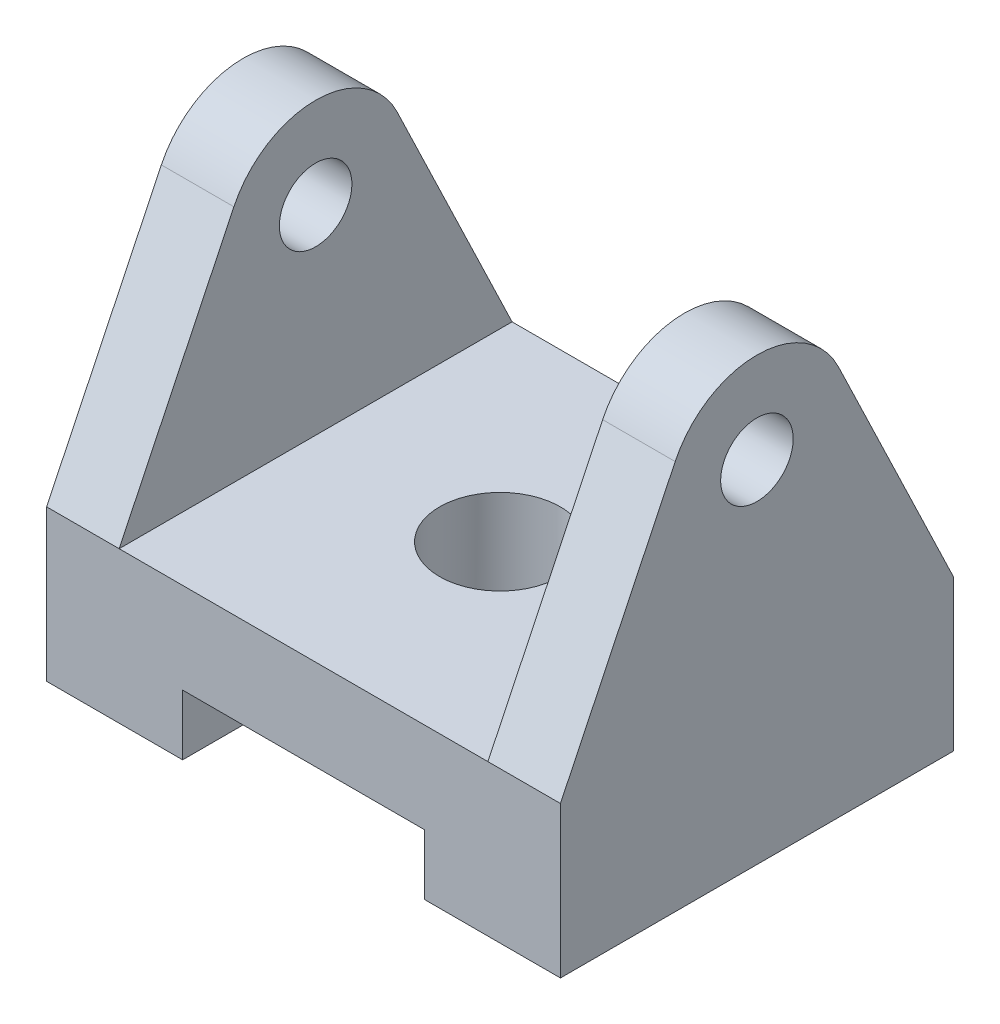
ISO-10303-21;
HEADER;
FILE_DESCRIPTION(('STEP AP214'),'2;1');
FILE_NAME('part.step','',(''),(''),'','','');
FILE_SCHEMA(('AUTOMOTIVE_DESIGN { 1 0 10303 214 1 1 1 1 }'));
ENDSEC;
DATA;
#1=APPLICATION_CONTEXT('core data for automotive mechanical design processes');
#2=APPLICATION_PROTOCOL_DEFINITION('international standard','automotive_design',2000,#1);
#3=PRODUCT_CONTEXT('',#1,'mechanical');
#4=PRODUCT('Part','Part','',(#3));
#5=PRODUCT_RELATED_PRODUCT_CATEGORY('part','',(#4));
#6=PRODUCT_DEFINITION_FORMATION('','',#4);
#7=PRODUCT_DEFINITION_CONTEXT('part definition',#1,'design');
#8=PRODUCT_DEFINITION('design','',#6,#7);
#9=PRODUCT_DEFINITION_SHAPE('','',#8);
#10=(LENGTH_UNIT() NAMED_UNIT(*) SI_UNIT(.MILLI.,.METRE.));
#11=(NAMED_UNIT(*) PLANE_ANGLE_UNIT() SI_UNIT($,.RADIAN.));
#12=(NAMED_UNIT(*) SI_UNIT($,.STERADIAN.) SOLID_ANGLE_UNIT());
#13=UNCERTAINTY_MEASURE_WITH_UNIT(LENGTH_MEASURE(1.E-05),#10,'distance_accuracy_value','');
#14=(GEOMETRIC_REPRESENTATION_CONTEXT(3) GLOBAL_UNCERTAINTY_ASSIGNED_CONTEXT((#13)) GLOBAL_UNIT_ASSIGNED_CONTEXT((#10,
#11,#12)) REPRESENTATION_CONTEXT('',''));
#15=CARTESIAN_POINT('',(0.,0.,0.));
#16=DIRECTION('',(0.,0.,1.));
#17=DIRECTION('',(1.,0.,0.));
#18=AXIS2_PLACEMENT_3D('',#15,#16,#17);
#19=CARTESIAN_POINT('',(30.5,29.,32.5));
#20=DIRECTION('',(1.,0.,0.));
#21=DIRECTION('',(0.,0.,-1.));
#22=AXIS2_PLACEMENT_3D('',#19,#20,#21);
#23=PLANE('',#22);
#24=CARTESIAN_POINT('',(30.5,29.,0.));
#25=DIRECTION('',(1.,0.,0.));
#26=DIRECTION('',(0.,1.,0.));
#27=AXIS2_PLACEMENT_3D('',#24,#25,#26);
#28=CIRCLE('',#27,6.);
#29=CARTESIAN_POINT('',(30.5,35.,0.));
#30=VERTEX_POINT('',#29);
#31=EDGE_CURVE('E193',#30,#30,#28,.T.);
#32=ORIENTED_EDGE('',*,*,#31,.T.);
#33=EDGE_LOOP('',(#32));
#34=FACE_BOUND('',#33,.T.);
#35=DIRECTION('',(0.,0.,-1.));
#36=VECTOR('',#35,1.);
#37=CARTESIAN_POINT('',(30.5,-4.,32.5));
#38=LINE('',#37,#36);
#39=CARTESIAN_POINT('',(30.5,-4.,32.5));
#40=VERTEX_POINT('',#39);
#41=CARTESIAN_POINT('',(30.5,-4.,-32.5));
#42=VERTEX_POINT('',#41);
#43=EDGE_CURVE('E51',#40,#42,#38,.T.);
#44=ORIENTED_EDGE('',*,*,#43,.F.);
#45=DIRECTION('',(0.,0.901331634338171,-0.433129639878502));
#46=VECTOR('',#45,1.);
#47=CARTESIAN_POINT('',(30.5,11.9373818614747,24.8413844546404));
#48=LINE('',#47,#46);
#49=CARTESIAN_POINT('',(30.5,35.4969445981775,13.5199745150726));
#50=VERTEX_POINT('',#49);
#51=EDGE_CURVE('E198',#40,#50,#48,.T.);
#52=ORIENTED_EDGE('',*,*,#51,.T.);
#53=CARTESIAN_POINT('',(30.5,29.,0.));
#54=DIRECTION('',(1.,0.,0.));
#55=DIRECTION('',(0.,1.,0.));
#56=AXIS2_PLACEMENT_3D('',#53,#54,#55);
#57=CIRCLE('',#56,15.);
#58=CARTESIAN_POINT('',(30.5,35.4969445981775,-13.5199745150726));
#59=VERTEX_POINT('',#58);
#60=EDGE_CURVE('E192',#59,#50,#57,.T.);
#61=ORIENTED_EDGE('',*,*,#60,.F.);
#62=DIRECTION('',(0.,0.901331634338171,0.433129639878502));
#63=VECTOR('',#62,1.);
#64=CARTESIAN_POINT('',(30.5,11.9373818614747,-24.8413844546404));
#65=LINE('',#64,#63);
#66=EDGE_CURVE('E186',#42,#59,#65,.T.);
#67=ORIENTED_EDGE('',*,*,#66,.F.);
#68=EDGE_LOOP('',(#44,#52,#61,#67));
#69=FACE_BOUND('',#68,.T.);
#70=ADVANCED_FACE('F41',(#34,#69),#23,.F.);
#71=CARTESIAN_POINT('',(-30.5,29.,32.5));
#72=DIRECTION('',(-1.,0.,0.));
#73=DIRECTION('',(0.,0.,1.));
#74=AXIS2_PLACEMENT_3D('',#71,#72,#73);
#75=PLANE('',#74);
#76=CARTESIAN_POINT('',(-30.5,29.,0.));
#77=DIRECTION('',(-1.,0.,0.));
#78=DIRECTION('',(0.,0.,1.));
#79=AXIS2_PLACEMENT_3D('',#76,#77,#78);
#80=CIRCLE('',#79,6.);
#81=CARTESIAN_POINT('',(-30.5,29.,6.));
#82=VERTEX_POINT('',#81);
#83=EDGE_CURVE('E203',#82,#82,#80,.T.);
#84=ORIENTED_EDGE('',*,*,#83,.T.);
#85=EDGE_LOOP('',(#84));
#86=FACE_BOUND('',#85,.T.);
#87=DIRECTION('',(0.,0.901331634338171,-0.433129639878502));
#88=VECTOR('',#87,1.);
#89=CARTESIAN_POINT('',(-30.5,11.9373818614747,24.8413844546404));
#90=LINE('',#89,#88);
#91=CARTESIAN_POINT('',(-30.5,-4.00000000000002,32.5));
#92=VERTEX_POINT('',#91);
#93=CARTESIAN_POINT('',(-30.5,35.4969445981775,13.5199745150726));
#94=VERTEX_POINT('',#93);
#95=EDGE_CURVE('E577',#92,#94,#90,.T.);
#96=ORIENTED_EDGE('',*,*,#95,.F.);
#97=DIRECTION('',(0.,0.,-1.));
#98=VECTOR('',#97,1.);
#99=CARTESIAN_POINT('',(-30.5,-4.,32.5));
#100=LINE('',#99,#98);
#101=CARTESIAN_POINT('',(-30.5,-4.,-32.5));
#102=VERTEX_POINT('',#101);
#103=EDGE_CURVE('E151',#92,#102,#100,.T.);
#104=ORIENTED_EDGE('',*,*,#103,.T.);
#105=DIRECTION('',(0.,0.901331634338172,0.433129639878502));
#106=VECTOR('',#105,1.);
#107=CARTESIAN_POINT('',(-30.5,11.9373818614747,-24.8413844546404));
#108=LINE('',#107,#106);
#109=CARTESIAN_POINT('',(-30.5,35.4969445981775,-13.5199745150726));
#110=VERTEX_POINT('',#109);
#111=EDGE_CURVE('E602',#102,#110,#108,.T.);
#112=ORIENTED_EDGE('',*,*,#111,.T.);
#113=CARTESIAN_POINT('',(-30.5,29.,0.));
#114=DIRECTION('',(-1.,0.,0.));
#115=DIRECTION('',(0.,-1.,0.));
#116=AXIS2_PLACEMENT_3D('',#113,#114,#115);
#117=CIRCLE('',#116,15.);
#118=EDGE_CURVE('E578',#110,#94,#117,.F.);
#119=ORIENTED_EDGE('',*,*,#118,.T.);
#120=EDGE_LOOP('',(#96,#104,#112,#119));
#121=FACE_BOUND('',#120,.T.);
#122=ADVANCED_FACE('F268',(#86,#121),#75,.F.);
#123=CARTESIAN_POINT('',(20.,-29.,32.5));
#124=DIRECTION('',(0.,1.,0.));
#125=DIRECTION('',(0.,0.,1.));
#126=AXIS2_PLACEMENT_3D('',#123,#124,#125);
#127=PLANE('',#126);
#128=DIRECTION('',(1.,0.,0.));
#129=VECTOR('',#128,1.);
#130=CARTESIAN_POINT('',(20.,-29.,-32.5));
#131=LINE('',#130,#129);
#132=CARTESIAN_POINT('',(20.,-29.,-32.5));
#133=VERTEX_POINT('',#132);
#134=CARTESIAN_POINT('',(42.5,-29.,-32.5));
#135=VERTEX_POINT('',#134);
#136=EDGE_CURVE('E131',#133,#135,#131,.T.);
#137=ORIENTED_EDGE('',*,*,#136,.T.);
#138=DIRECTION('',(0.,0.,-1.));
#139=VECTOR('',#138,1.);
#140=CARTESIAN_POINT('',(42.5,-29.,32.5));
#141=LINE('',#140,#139);
#142=CARTESIAN_POINT('',(42.5,-29.,32.5));
#143=VERTEX_POINT('',#142);
#144=EDGE_CURVE('E11',#143,#135,#141,.T.);
#145=ORIENTED_EDGE('',*,*,#144,.F.);
#146=DIRECTION('',(1.,0.,0.));
#147=VECTOR('',#146,1.);
#148=CARTESIAN_POINT('',(20.,-29.,32.5));
#149=LINE('',#148,#147);
#150=CARTESIAN_POINT('',(20.,-29.,32.5));
#151=VERTEX_POINT('',#150);
#152=EDGE_CURVE('E147',#151,#143,#149,.T.);
#153=ORIENTED_EDGE('',*,*,#152,.F.);
#154=DIRECTION('',(0.,0.,-1.));
#155=VECTOR('',#154,1.);
#156=CARTESIAN_POINT('',(20.,-29.,32.5));
#157=LINE('',#156,#155);
#158=EDGE_CURVE('E126',#151,#133,#157,.T.);
#159=ORIENTED_EDGE('',*,*,#158,.T.);
#160=EDGE_LOOP('',(#137,#145,#153,#159));
#161=FACE_BOUND('',#160,.T.);
#162=ADVANCED_FACE('F43',(#161),#127,.F.);
#163=CARTESIAN_POINT('',(42.5,29.,32.5));
#164=DIRECTION('',(-1.,0.,0.));
#165=DIRECTION('',(0.,-1.,0.));
#166=AXIS2_PLACEMENT_3D('',#163,#164,#165);
#167=PLANE('',#166);
#168=DIRECTION('',(0.,0.901331634338171,-0.433129639878502));
#169=VECTOR('',#168,1.);
#170=CARTESIAN_POINT('',(42.5,11.9373818614747,24.8413844546404));
#171=LINE('',#170,#169);
#172=CARTESIAN_POINT('',(42.5,-4.,32.5));
#173=VERTEX_POINT('',#172);
#174=CARTESIAN_POINT('',(42.5,35.4969445981775,13.5199745150726));
#175=VERTEX_POINT('',#174);
#176=EDGE_CURVE('E222',#173,#175,#171,.T.);
#177=ORIENTED_EDGE('',*,*,#176,.F.);
#178=DIRECTION('',(0.,1.,0.));
#179=VECTOR('',#178,1.);
#180=CARTESIAN_POINT('',(42.5,29.,32.5));
#181=LINE('',#180,#179);
#182=EDGE_CURVE('E97',#143,#173,#181,.T.);
#183=ORIENTED_EDGE('',*,*,#182,.F.);
#184=ORIENTED_EDGE('',*,*,#144,.T.);
#185=DIRECTION('',(0.,1.,0.));
#186=VECTOR('',#185,1.);
#187=CARTESIAN_POINT('',(42.5,29.,-32.5));
#188=LINE('',#187,#186);
#189=CARTESIAN_POINT('',(42.5,-4.,-32.5));
#190=VERTEX_POINT('',#189);
#191=EDGE_CURVE('E137',#135,#190,#188,.T.);
#192=ORIENTED_EDGE('',*,*,#191,.T.);
#193=DIRECTION('',(0.,0.901331634338171,0.433129639878502));
#194=VECTOR('',#193,1.);
#195=CARTESIAN_POINT('',(42.5,11.9373818614747,-24.8413844546404));
#196=LINE('',#195,#194);
#197=CARTESIAN_POINT('',(42.5,35.4969445981775,-13.5199745150726));
#198=VERTEX_POINT('',#197);
#199=EDGE_CURVE('E202',#190,#198,#196,.T.);
#200=ORIENTED_EDGE('',*,*,#199,.T.);
#201=CARTESIAN_POINT('',(42.5,29.,0.));
#202=DIRECTION('',(1.,0.,0.));
#203=DIRECTION('',(0.,1.,0.));
#204=AXIS2_PLACEMENT_3D('',#201,#202,#203);
#205=CIRCLE('',#204,15.);
#206=EDGE_CURVE('E207',#198,#175,#205,.T.);
#207=ORIENTED_EDGE('',*,*,#206,.T.);
#208=EDGE_LOOP('',(#177,#183,#184,#192,#200,#207));
#209=FACE_BOUND('',#208,.T.);
#210=CARTESIAN_POINT('',(42.5,29.,0.));
#211=DIRECTION('',(1.,0.,0.));
#212=DIRECTION('',(0.,1.,0.));
#213=AXIS2_PLACEMENT_3D('',#210,#211,#212);
#214=CIRCLE('',#213,6.);
#215=CARTESIAN_POINT('',(42.5,35.,0.));
#216=VERTEX_POINT('',#215);
#217=EDGE_CURVE('E211',#216,#216,#214,.T.);
#218=ORIENTED_EDGE('',*,*,#217,.F.);
#219=EDGE_LOOP('',(#218));
#220=FACE_BOUND('',#219,.T.);
#221=ADVANCED_FACE('F279',(#209,#220),#167,.F.);
#222=CARTESIAN_POINT('',(30.5,-4.,32.5));
#223=DIRECTION('',(0.,-1.,0.));
#224=DIRECTION('',(0.,0.,-1.));
#225=AXIS2_PLACEMENT_3D('',#222,#223,#224);
#226=PLANE('',#225);
#227=CARTESIAN_POINT('',(0.,-4.,0.));
#228=DIRECTION('',(0.,1.,0.));
#229=DIRECTION('',(0.,0.,1.));
#230=AXIS2_PLACEMENT_3D('',#227,#228,#229);
#231=CIRCLE('',#230,10.);
#232=CARTESIAN_POINT('',(0.,-4.,10.));
#233=VERTEX_POINT('',#232);
#234=EDGE_CURVE('E230',#233,#233,#231,.T.);
#235=ORIENTED_EDGE('',*,*,#234,.F.);
#236=EDGE_LOOP('',(#235));
#237=FACE_BOUND('',#236,.T.);
#238=ORIENTED_EDGE('',*,*,#103,.F.);
#239=DIRECTION('',(1.,0.,0.));
#240=VECTOR('',#239,1.);
#241=CARTESIAN_POINT('',(-30.5,-4.,32.5));
#242=LINE('',#241,#240);
#243=EDGE_CURVE('E169',#92,#40,#242,.T.);
#244=ORIENTED_EDGE('',*,*,#243,.T.);
#245=ORIENTED_EDGE('',*,*,#43,.T.);
#246=DIRECTION('',(-1.,0.,0.));
#247=VECTOR('',#246,1.);
#248=CARTESIAN_POINT('',(-30.5,-4.,-32.5));
#249=LINE('',#248,#247);
#250=EDGE_CURVE('E168',#42,#102,#249,.T.);
#251=ORIENTED_EDGE('',*,*,#250,.T.);
#252=EDGE_LOOP('',(#238,#244,#245,#251));
#253=FACE_BOUND('',#252,.T.);
#254=ADVANCED_FACE('F165',(#237,#253),#226,.F.);
#255=CARTESIAN_POINT('',(-42.5,29.,32.5));
#256=DIRECTION('',(1.,0.,0.));
#257=DIRECTION('',(0.,1.,0.));
#258=AXIS2_PLACEMENT_3D('',#255,#256,#257);
#259=PLANE('',#258);
#260=CARTESIAN_POINT('',(-42.5,29.,0.));
#261=DIRECTION('',(1.,0.,0.));
#262=DIRECTION('',(0.,1.,0.));
#263=AXIS2_PLACEMENT_3D('',#260,#261,#262);
#264=CIRCLE('',#263,6.);
#265=CARTESIAN_POINT('',(-42.5,35.,0.));
#266=VERTEX_POINT('',#265);
#267=EDGE_CURVE('E209',#266,#266,#264,.T.);
#268=ORIENTED_EDGE('',*,*,#267,.T.);
#269=EDGE_LOOP('',(#268));
#270=FACE_BOUND('',#269,.T.);
#271=DIRECTION('',(0.,0.901331634338171,-0.433129639878502));
#272=VECTOR('',#271,1.);
#273=CARTESIAN_POINT('',(-42.5,11.9373818614747,24.8413844546404));
#274=LINE('',#273,#272);
#275=CARTESIAN_POINT('',(-42.5,-4.00000000000002,32.5));
#276=VERTEX_POINT('',#275);
#277=CARTESIAN_POINT('',(-42.5,35.4969445981775,13.5199745150726));
#278=VERTEX_POINT('',#277);
#279=EDGE_CURVE('E583',#276,#278,#274,.T.);
#280=ORIENTED_EDGE('',*,*,#279,.T.);
#281=CARTESIAN_POINT('',(-42.5,29.,0.));
#282=DIRECTION('',(-1.,0.,0.));
#283=DIRECTION('',(0.,-1.,0.));
#284=AXIS2_PLACEMENT_3D('',#281,#282,#283);
#285=CIRCLE('',#284,15.);
#286=CARTESIAN_POINT('',(-42.5,35.4969445981775,-13.5199745150726));
#287=VERTEX_POINT('',#286);
#288=EDGE_CURVE('E184',#287,#278,#285,.F.);
#289=ORIENTED_EDGE('',*,*,#288,.F.);
#290=DIRECTION('',(0.,0.901331634338172,0.433129639878502));
#291=VECTOR('',#290,1.);
#292=CARTESIAN_POINT('',(-42.5,11.9373818614747,-24.8413844546404));
#293=LINE('',#292,#291);
#294=CARTESIAN_POINT('',(-42.5,-4.00000000000002,-32.5));
#295=VERTEX_POINT('',#294);
#296=EDGE_CURVE('E598',#295,#287,#293,.T.);
#297=ORIENTED_EDGE('',*,*,#296,.F.);
#298=DIRECTION('',(0.,-1.,0.));
#299=VECTOR('',#298,1.);
#300=CARTESIAN_POINT('',(-42.5,29.,-32.5));
#301=LINE('',#300,#299);
#302=CARTESIAN_POINT('',(-42.5,-29.,-32.5));
#303=VERTEX_POINT('',#302);
#304=EDGE_CURVE('E139',#295,#303,#301,.T.);
#305=ORIENTED_EDGE('',*,*,#304,.T.);
#306=DIRECTION('',(0.,0.,-1.));
#307=VECTOR('',#306,1.);
#308=CARTESIAN_POINT('',(-42.5,-29.,32.5));
#309=LINE('',#308,#307);
#310=CARTESIAN_POINT('',(-42.5,-29.,32.5));
#311=VERTEX_POINT('',#310);
#312=EDGE_CURVE('E148',#311,#303,#309,.T.);
#313=ORIENTED_EDGE('',*,*,#312,.F.);
#314=DIRECTION('',(0.,-1.,0.));
#315=VECTOR('',#314,1.);
#316=CARTESIAN_POINT('',(-42.5,29.,32.5));
#317=LINE('',#316,#315);
#318=EDGE_CURVE('E236',#276,#311,#317,.T.);
#319=ORIENTED_EDGE('',*,*,#318,.F.);
#320=EDGE_LOOP('',(#280,#289,#297,#305,#313,#319));
#321=FACE_BOUND('',#320,.T.);
#322=ADVANCED_FACE('F246',(#270,#321),#259,.F.);
#323=CARTESIAN_POINT('',(-42.5,-29.,32.5));
#324=DIRECTION('',(0.,1.,0.));
#325=DIRECTION('',(0.,0.,1.));
#326=AXIS2_PLACEMENT_3D('',#323,#324,#325);
#327=PLANE('',#326);
#328=DIRECTION('',(1.,0.,0.));
#329=VECTOR('',#328,1.);
#330=CARTESIAN_POINT('',(-42.5,-29.,-32.5));
#331=LINE('',#330,#329);
#332=CARTESIAN_POINT('',(-20.,-29.,-32.5));
#333=VERTEX_POINT('',#332);
#334=EDGE_CURVE('E142',#303,#333,#331,.T.);
#335=ORIENTED_EDGE('',*,*,#334,.T.);
#336=DIRECTION('',(0.,0.,-1.));
#337=VECTOR('',#336,1.);
#338=CARTESIAN_POINT('',(-20.,-29.,32.5));
#339=LINE('',#338,#337);
#340=CARTESIAN_POINT('',(-20.,-29.,32.5));
#341=VERTEX_POINT('',#340);
#342=EDGE_CURVE('E121',#341,#333,#339,.T.);
#343=ORIENTED_EDGE('',*,*,#342,.F.);
#344=DIRECTION('',(1.,0.,0.));
#345=VECTOR('',#344,1.);
#346=CARTESIAN_POINT('',(-42.5,-29.,32.5));
#347=LINE('',#346,#345);
#348=EDGE_CURVE('E114',#311,#341,#347,.T.);
#349=ORIENTED_EDGE('',*,*,#348,.F.);
#350=ORIENTED_EDGE('',*,*,#312,.T.);
#351=EDGE_LOOP('',(#335,#343,#349,#350));
#352=FACE_BOUND('',#351,.T.);
#353=ADVANCED_FACE('F249',(#352),#327,.F.);
#354=CARTESIAN_POINT('',(-20.,-19.,32.5));
#355=DIRECTION('',(-1.,0.,0.));
#356=DIRECTION('',(0.,0.,1.));
#357=AXIS2_PLACEMENT_3D('',#354,#355,#356);
#358=PLANE('',#357);
#359=DIRECTION('',(0.,1.,0.));
#360=VECTOR('',#359,1.);
#361=CARTESIAN_POINT('',(-20.,-19.,-32.5));
#362=LINE('',#361,#360);
#363=CARTESIAN_POINT('',(-20.,-19.,-32.5));
#364=VERTEX_POINT('',#363);
#365=EDGE_CURVE('E124',#333,#364,#362,.T.);
#366=ORIENTED_EDGE('',*,*,#365,.T.);
#367=DIRECTION('',(0.,0.,-1.));
#368=VECTOR('',#367,1.);
#369=CARTESIAN_POINT('',(-20.,-19.,32.5));
#370=LINE('',#369,#368);
#371=CARTESIAN_POINT('',(-20.,-19.,32.5));
#372=VERTEX_POINT('',#371);
#373=EDGE_CURVE('E119',#372,#364,#370,.T.);
#374=ORIENTED_EDGE('',*,*,#373,.F.);
#375=DIRECTION('',(0.,1.,0.));
#376=VECTOR('',#375,1.);
#377=CARTESIAN_POINT('',(-20.,-19.,32.5));
#378=LINE('',#377,#376);
#379=EDGE_CURVE('E108',#341,#372,#378,.T.);
#380=ORIENTED_EDGE('',*,*,#379,.F.);
#381=ORIENTED_EDGE('',*,*,#342,.T.);
#382=EDGE_LOOP('',(#366,#374,#380,#381));
#383=FACE_BOUND('',#382,.T.);
#384=ADVANCED_FACE('F122',(#383),#358,.F.);
#385=CARTESIAN_POINT('',(20.,-19.,32.5));
#386=DIRECTION('',(0.,1.,0.));
#387=DIRECTION('',(-1.,0.,0.));
#388=AXIS2_PLACEMENT_3D('',#385,#386,#387);
#389=PLANE('',#388);
#390=CARTESIAN_POINT('',(0.,-19.,0.));
#391=DIRECTION('',(0.,1.,0.));
#392=DIRECTION('',(-1.,0.,0.));
#393=AXIS2_PLACEMENT_3D('',#390,#391,#392);
#394=CIRCLE('',#393,10.);
#395=CARTESIAN_POINT('',(-10.,-19.,0.));
#396=VERTEX_POINT('',#395);
#397=EDGE_CURVE('E44',#396,#396,#394,.T.);
#398=ORIENTED_EDGE('',*,*,#397,.T.);
#399=EDGE_LOOP('',(#398));
#400=FACE_BOUND('',#399,.T.);
#401=DIRECTION('',(1.,0.,0.));
#402=VECTOR('',#401,1.);
#403=CARTESIAN_POINT('',(20.,-19.,-32.5));
#404=LINE('',#403,#402);
#405=CARTESIAN_POINT('',(20.,-19.,-32.5));
#406=VERTEX_POINT('',#405);
#407=EDGE_CURVE('E84',#364,#406,#404,.T.);
#408=ORIENTED_EDGE('',*,*,#407,.T.);
#409=DIRECTION('',(0.,0.,-1.));
#410=VECTOR('',#409,1.);
#411=CARTESIAN_POINT('',(20.,-19.,32.5));
#412=LINE('',#411,#410);
#413=CARTESIAN_POINT('',(20.,-19.,32.5));
#414=VERTEX_POINT('',#413);
#415=EDGE_CURVE('E123',#414,#406,#412,.T.);
#416=ORIENTED_EDGE('',*,*,#415,.F.);
#417=DIRECTION('',(1.,0.,0.));
#418=VECTOR('',#417,1.);
#419=CARTESIAN_POINT('',(20.,-19.,32.5));
#420=LINE('',#419,#418);
#421=EDGE_CURVE('E113',#372,#414,#420,.T.);
#422=ORIENTED_EDGE('',*,*,#421,.F.);
#423=ORIENTED_EDGE('',*,*,#373,.T.);
#424=EDGE_LOOP('',(#408,#416,#422,#423));
#425=FACE_BOUND('',#424,.T.);
#426=ADVANCED_FACE('F130',(#400,#425),#389,.F.);
#427=CARTESIAN_POINT('',(20.,-29.,32.5));
#428=DIRECTION('',(1.,0.,0.));
#429=DIRECTION('',(0.,0.,-1.));
#430=AXIS2_PLACEMENT_3D('',#427,#428,#429);
#431=PLANE('',#430);
#432=DIRECTION('',(0.,-1.,0.));
#433=VECTOR('',#432,1.);
#434=CARTESIAN_POINT('',(20.,-29.,-32.5));
#435=LINE('',#434,#433);
#436=EDGE_CURVE('E87',#406,#133,#435,.T.);
#437=ORIENTED_EDGE('',*,*,#436,.T.);
#438=ORIENTED_EDGE('',*,*,#158,.F.);
#439=DIRECTION('',(0.,-1.,0.));
#440=VECTOR('',#439,1.);
#441=CARTESIAN_POINT('',(20.,-29.,32.5));
#442=LINE('',#441,#440);
#443=EDGE_CURVE('E56',#414,#151,#442,.T.);
#444=ORIENTED_EDGE('',*,*,#443,.F.);
#445=ORIENTED_EDGE('',*,*,#415,.T.);
#446=EDGE_LOOP('',(#437,#438,#444,#445));
#447=FACE_BOUND('',#446,.T.);
#448=ADVANCED_FACE('F253',(#447),#431,.F.);
#449=CARTESIAN_POINT('',(0.,0.,32.5));
#450=DIRECTION('',(0.,0.,-1.));
#451=DIRECTION('',(-1.,0.,0.));
#452=AXIS2_PLACEMENT_3D('',#449,#450,#451);
#453=PLANE('',#452);
#454=ORIENTED_EDGE('',*,*,#243,.F.);
#455=DIRECTION('',(-1.,0.,0.));
#456=VECTOR('',#455,1.);
#457=CARTESIAN_POINT('',(-30.5,-4.00000000000002,32.5));
#458=LINE('',#457,#456);
#459=EDGE_CURVE('E245',#92,#276,#458,.T.);
#460=ORIENTED_EDGE('',*,*,#459,.T.);
#461=ORIENTED_EDGE('',*,*,#318,.T.);
#462=ORIENTED_EDGE('',*,*,#348,.T.);
#463=ORIENTED_EDGE('',*,*,#379,.T.);
#464=ORIENTED_EDGE('',*,*,#421,.T.);
#465=ORIENTED_EDGE('',*,*,#443,.T.);
#466=ORIENTED_EDGE('',*,*,#152,.T.);
#467=ORIENTED_EDGE('',*,*,#182,.T.);
#468=DIRECTION('',(1.,0.,0.));
#469=VECTOR('',#468,1.);
#470=CARTESIAN_POINT('',(30.5,-4.,32.5));
#471=LINE('',#470,#469);
#472=EDGE_CURVE('E205',#40,#173,#471,.T.);
#473=ORIENTED_EDGE('',*,*,#472,.F.);
#474=EDGE_LOOP('',(#454,#460,#461,#462,#463,#464,#465,#466,#467,#473));
#475=FACE_BOUND('',#474,.T.);
#476=ADVANCED_FACE('F111',(#475),#453,.F.);
#477=CARTESIAN_POINT('',(0.,0.,-32.5));
#478=DIRECTION('',(0.,0.,-1.));
#479=DIRECTION('',(-1.,0.,0.));
#480=AXIS2_PLACEMENT_3D('',#477,#478,#479);
#481=PLANE('',#480);
#482=DIRECTION('',(-1.,0.,0.));
#483=VECTOR('',#482,1.);
#484=CARTESIAN_POINT('',(-30.5,-4.00000000000002,-32.5));
#485=LINE('',#484,#483);
#486=EDGE_CURVE('E182',#102,#295,#485,.T.);
#487=ORIENTED_EDGE('',*,*,#486,.F.);
#488=ORIENTED_EDGE('',*,*,#250,.F.);
#489=DIRECTION('',(1.,0.,0.));
#490=VECTOR('',#489,1.);
#491=CARTESIAN_POINT('',(30.5,-4.,-32.5));
#492=LINE('',#491,#490);
#493=EDGE_CURVE('E179',#42,#190,#492,.T.);
#494=ORIENTED_EDGE('',*,*,#493,.T.);
#495=ORIENTED_EDGE('',*,*,#191,.F.);
#496=ORIENTED_EDGE('',*,*,#136,.F.);
#497=ORIENTED_EDGE('',*,*,#436,.F.);
#498=ORIENTED_EDGE('',*,*,#407,.F.);
#499=ORIENTED_EDGE('',*,*,#365,.F.);
#500=ORIENTED_EDGE('',*,*,#334,.F.);
#501=ORIENTED_EDGE('',*,*,#304,.F.);
#502=EDGE_LOOP('',(#487,#488,#494,#495,#496,#497,#498,#499,#500,#501));
#503=FACE_BOUND('',#502,.T.);
#504=ADVANCED_FACE('F180',(#503),#481,.T.);
#505=CARTESIAN_POINT('',(0.,-69.,0.));
#506=DIRECTION('',(0.,1.,0.));
#507=DIRECTION('',(0.,0.,1.));
#508=AXIS2_PLACEMENT_3D('',#505,#506,#507);
#509=CYLINDRICAL_SURFACE('',#508,10.);
#510=ORIENTED_EDGE('',*,*,#234,.T.);
#511=EDGE_LOOP('',(#510));
#512=FACE_BOUND('',#511,.T.);
#513=ORIENTED_EDGE('',*,*,#397,.F.);
#514=EDGE_LOOP('',(#513));
#515=FACE_BOUND('',#514,.T.);
#516=ADVANCED_FACE('F295',(#512,#515),#509,.F.);
#517=CARTESIAN_POINT('',(30.5,29.,0.));
#518=DIRECTION('',(1.,0.,0.));
#519=DIRECTION('',(0.,1.,0.));
#520=AXIS2_PLACEMENT_3D('',#517,#518,#519);
#521=CYLINDRICAL_SURFACE('',#520,6.);
#522=ORIENTED_EDGE('',*,*,#217,.T.);
#523=EDGE_LOOP('',(#522));
#524=FACE_BOUND('',#523,.T.);
#525=ORIENTED_EDGE('',*,*,#31,.F.);
#526=EDGE_LOOP('',(#525));
#527=FACE_BOUND('',#526,.T.);
#528=ADVANCED_FACE('F293',(#524,#527),#521,.F.);
#529=CARTESIAN_POINT('',(30.5,11.9373818614747,24.8413844546404));
#530=DIRECTION('',(0.,-0.433129639878502,-0.901331634338171));
#531=DIRECTION('',(0.,0.901331634338171,-0.433129639878502));
#532=AXIS2_PLACEMENT_3D('',#529,#530,#531);
#533=PLANE('',#532);
#534=ORIENTED_EDGE('',*,*,#51,.F.);
#535=ORIENTED_EDGE('',*,*,#472,.T.);
#536=ORIENTED_EDGE('',*,*,#176,.T.);
#537=DIRECTION('',(1.,0.,0.));
#538=VECTOR('',#537,1.);
#539=CARTESIAN_POINT('',(30.5,35.4969445981775,13.5199745150726));
#540=LINE('',#539,#538);
#541=EDGE_CURVE('E216',#50,#175,#540,.T.);
#542=ORIENTED_EDGE('',*,*,#541,.F.);
#543=EDGE_LOOP('',(#534,#535,#536,#542));
#544=FACE_BOUND('',#543,.T.);
#545=ADVANCED_FACE('F291',(#544),#533,.F.);
#546=CARTESIAN_POINT('',(30.5,11.9373818614747,-24.8413844546404));
#547=DIRECTION('',(0.,0.433129639878502,-0.901331634338171));
#548=DIRECTION('',(0.,0.901331634338171,0.433129639878502));
#549=AXIS2_PLACEMENT_3D('',#546,#547,#548);
#550=PLANE('',#549);
#551=ORIENTED_EDGE('',*,*,#199,.F.);
#552=ORIENTED_EDGE('',*,*,#493,.F.);
#553=ORIENTED_EDGE('',*,*,#66,.T.);
#554=DIRECTION('',(1.,0.,0.));
#555=VECTOR('',#554,1.);
#556=CARTESIAN_POINT('',(30.5,35.4969445981775,-13.5199745150726));
#557=LINE('',#556,#555);
#558=EDGE_CURVE('E227',#59,#198,#557,.T.);
#559=ORIENTED_EDGE('',*,*,#558,.T.);
#560=EDGE_LOOP('',(#551,#552,#553,#559));
#561=FACE_BOUND('',#560,.T.);
#562=ADVANCED_FACE('F197',(#561),#550,.T.);
#563=CARTESIAN_POINT('',(30.5,29.,0.));
#564=DIRECTION('',(1.,0.,0.));
#565=DIRECTION('',(0.,1.,0.));
#566=AXIS2_PLACEMENT_3D('',#563,#564,#565);
#567=CYLINDRICAL_SURFACE('',#566,15.);
#568=ORIENTED_EDGE('',*,*,#206,.F.);
#569=ORIENTED_EDGE('',*,*,#558,.F.);
#570=ORIENTED_EDGE('',*,*,#60,.T.);
#571=ORIENTED_EDGE('',*,*,#541,.T.);
#572=EDGE_LOOP('',(#568,#569,#570,#571));
#573=FACE_BOUND('',#572,.T.);
#574=ADVANCED_FACE('F311',(#573),#567,.T.);
#575=CARTESIAN_POINT('',(-42.5,29.,0.));
#576=DIRECTION('',(1.,0.,0.));
#577=DIRECTION('',(0.,1.,0.));
#578=AXIS2_PLACEMENT_3D('',#575,#576,#577);
#579=CYLINDRICAL_SURFACE('',#578,6.);
#580=ORIENTED_EDGE('',*,*,#267,.F.);
#581=EDGE_LOOP('',(#580));
#582=FACE_BOUND('',#581,.T.);
#583=ORIENTED_EDGE('',*,*,#83,.F.);
#584=EDGE_LOOP('',(#583));
#585=FACE_BOUND('',#584,.T.);
#586=ADVANCED_FACE('F308',(#582,#585),#579,.F.);
#587=CARTESIAN_POINT('',(-30.5,11.9373818614747,-24.8413844546404));
#588=DIRECTION('',(0.,-0.433129639878502,0.901331634338171));
#589=DIRECTION('',(0.,-0.901331634338172,-0.433129639878502));
#590=AXIS2_PLACEMENT_3D('',#587,#588,#589);
#591=PLANE('',#590);
#592=ORIENTED_EDGE('',*,*,#296,.T.);
#593=DIRECTION('',(-1.,0.,0.));
#594=VECTOR('',#593,1.);
#595=CARTESIAN_POINT('',(-30.5,35.4969445981775,-13.5199745150726));
#596=LINE('',#595,#594);
#597=EDGE_CURVE('E594',#110,#287,#596,.T.);
#598=ORIENTED_EDGE('',*,*,#597,.F.);
#599=ORIENTED_EDGE('',*,*,#111,.F.);
#600=ORIENTED_EDGE('',*,*,#486,.T.);
#601=EDGE_LOOP('',(#592,#598,#599,#600));
#602=FACE_BOUND('',#601,.T.);
#603=ADVANCED_FACE('F333',(#602),#591,.F.);
#604=CARTESIAN_POINT('',(-30.5,11.9373818614747,24.8413844546404));
#605=DIRECTION('',(0.,0.433129639878502,0.901331634338171));
#606=DIRECTION('',(0.,-0.901331634338171,0.433129639878502));
#607=AXIS2_PLACEMENT_3D('',#604,#605,#606);
#608=PLANE('',#607);
#609=ORIENTED_EDGE('',*,*,#279,.F.);
#610=ORIENTED_EDGE('',*,*,#459,.F.);
#611=ORIENTED_EDGE('',*,*,#95,.T.);
#612=DIRECTION('',(-1.,0.,0.));
#613=VECTOR('',#612,1.);
#614=CARTESIAN_POINT('',(-30.5,35.4969445981775,13.5199745150726));
#615=LINE('',#614,#613);
#616=EDGE_CURVE('E592',#94,#278,#615,.T.);
#617=ORIENTED_EDGE('',*,*,#616,.T.);
#618=EDGE_LOOP('',(#609,#610,#611,#617));
#619=FACE_BOUND('',#618,.T.);
#620=ADVANCED_FACE('F337',(#619),#608,.T.);
#621=CARTESIAN_POINT('',(-30.5,29.,0.));
#622=DIRECTION('',(-1.,0.,0.));
#623=DIRECTION('',(0.,-1.,0.));
#624=AXIS2_PLACEMENT_3D('',#621,#622,#623);
#625=CYLINDRICAL_SURFACE('',#624,15.);
#626=ORIENTED_EDGE('',*,*,#288,.T.);
#627=ORIENTED_EDGE('',*,*,#616,.F.);
#628=ORIENTED_EDGE('',*,*,#118,.F.);
#629=ORIENTED_EDGE('',*,*,#597,.T.);
#630=EDGE_LOOP('',(#626,#627,#628,#629));
#631=FACE_BOUND('',#630,.T.);
#632=ADVANCED_FACE('F324',(#631),#625,.T.);
#633=CLOSED_SHELL('',(#70,#122,#162,#221,#254,#322,#353,#384,#426,#448,#476,#504,#516,#528,#545,
#562,#574,#586,#603,#620,#632));
#634=MANIFOLD_SOLID_BREP('B2',#633);
#635=ADVANCED_BREP_SHAPE_REPRESENTATION('',(#18,#634),#14);
#636=SHAPE_DEFINITION_REPRESENTATION(#9,#635);
ENDSEC;
END-ISO-10303-21;
